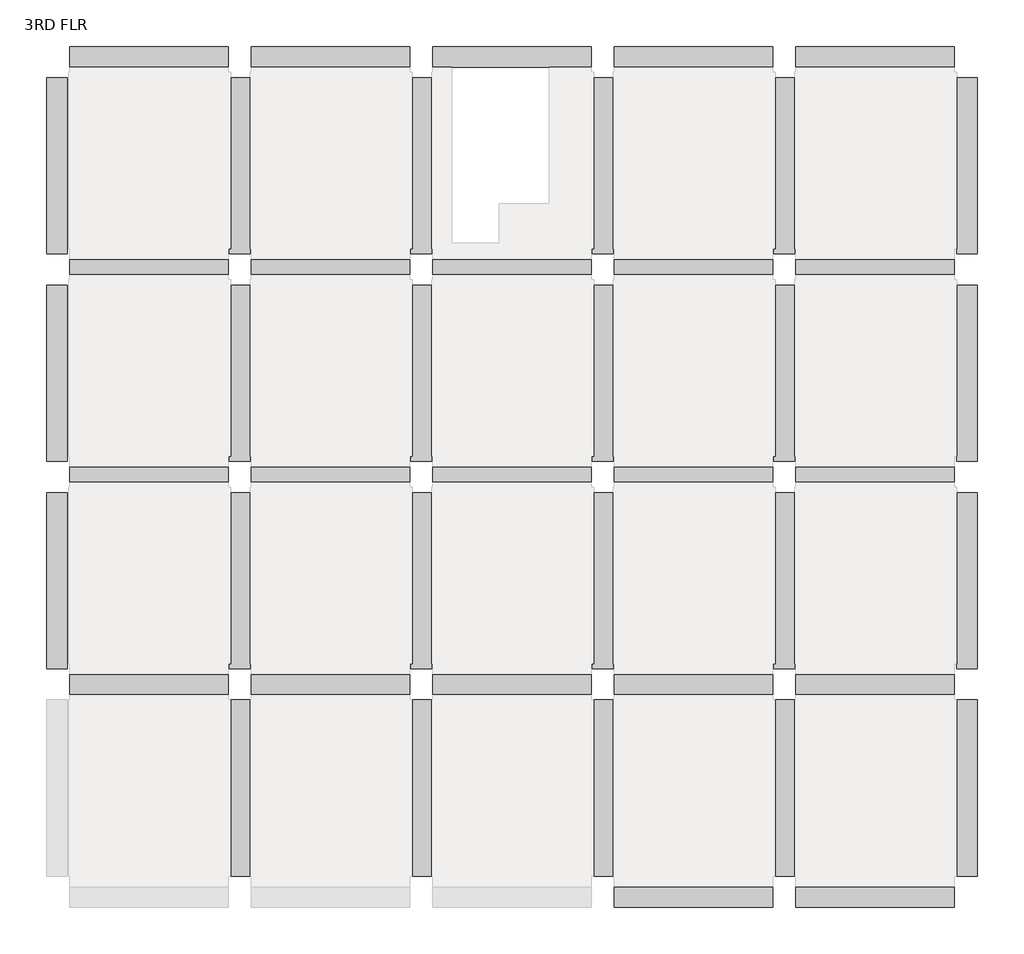
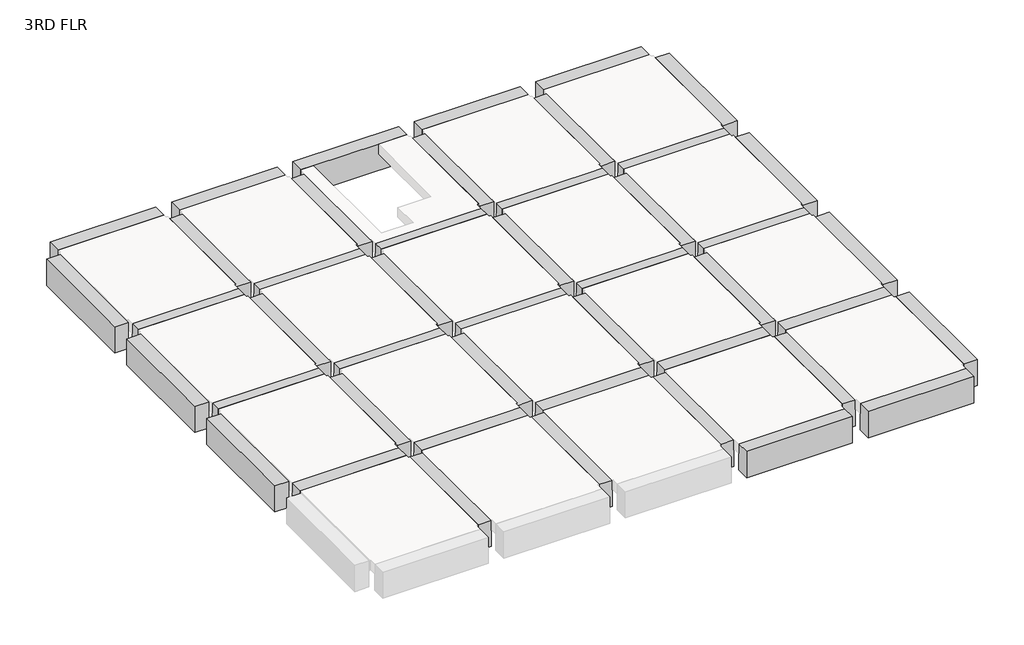
# One storey, part 2 of 2: 45 beams.
"""IFC4 building model written with IfcOpenShell, lengths in millimetres."""

from ifc_helpers import new_model, si_unit, frame, origin, place, context, project, spatial, polyline, outline, extrude, faceted_brep, element, save

model = new_model("IFC4")

# Units and contexts
model_context = context("Model", 3, world=origin())
ifc_project = project(units=[si_unit("LENGTHUNIT", "METRE", prefix="MILLI")], contexts=[model_context])

# Site, building, storey
site = spatial("IfcSite", under=ifc_project)
building = spatial("IfcBuilding", under=site)
storey = spatial("IfcBuildingStorey", under=building, Name="3RD FLR", Elevation=9144.0)

# Beams
placement = place(None, origin())
element("IfcBeam", 1, ObjectType="M_Concrete-Rectangular Beam : 400 x 800mm", at=placement, inside=storey, context=model_context, shape_type="Brep", body=[
    faceted_brep([(7955.1115906, 15703.1212443, 9144.0), (8355.1115906, 15703.1212443, 9144.0), (8355.1115906, 19103.1212443, 9144.0), (7955.1115906, 19103.1212443, 9144.0), (7955.1115906, 15803.1212443, 9144.0), (7955.1115906, 15703.1212443, 8344.0), (7955.1115906, 19103.1212443, 8344.0), (8355.1115906, 15703.1212443, 8344.0), (8355.1115906, 19103.1212443, 8344.0)], [[[0, 1, 2, 3, 4]], [[5, 0, 4, 3, 6]], [[7, 5, 6, 8]], [[1, 7, 8, 2]], [[2, 8, 6, 3]], [[1, 0, 5, 7]]]),
])
element("IfcBeam", 2, ObjectType="M_Concrete-Rectangular Beam : 400 x 800mm", at=placement, inside=storey, context=model_context, shape_type="Brep", body=[
    faceted_brep([(7955.1115906, 11703.1212443, 9144.0), (8355.1115906, 11703.1212443, 9144.0), (8355.1115906, 15103.1212443, 9144.0), (7955.1115906, 15103.1212443, 9144.0), (7955.1115906, 11803.1212443, 9144.0), (7955.1115906, 11703.1212443, 8344.0), (7955.1115906, 15103.1212443, 8344.0), (8355.1115906, 11703.1212443, 8344.0), (8355.1115906, 15103.1212443, 8344.0)], [[[0, 1, 2, 3, 4]], [[5, 0, 4, 3, 6]], [[7, 5, 6, 8]], [[1, 7, 8, 2]], [[2, 8, 6, 3]], [[1, 0, 5, 7]]]),
])
element("IfcBeam", 3, ObjectType="M_Concrete-Rectangular Beam : 400 x 800mm", at=placement, inside=storey, context=model_context, shape_type="Brep", body=[
    faceted_brep([(7955.1115906, 7703.1212443, 9144.0), (8355.1115906, 7703.1212443, 9144.0), (8355.1115906, 11103.1212443, 9144.0), (7955.1115906, 11103.1212443, 9144.0), (7955.1115906, 7803.1212443, 9144.0), (7955.1115906, 7703.1212443, 8344.0), (7955.1115906, 11103.1212443, 8344.0), (8355.1115906, 7703.1212443, 8344.0), (8355.1115906, 11103.1212443, 8344.0)], [[[0, 1, 2, 3, 4]], [[5, 0, 4, 3, 6]], [[7, 5, 6, 8]], [[1, 7, 8, 2]], [[1, 0, 5, 7]], [[3, 2, 8, 6]]]),
])
element("IfcBeam", 4, ObjectType="M_Concrete-Rectangular Beam : 400 x 800mm", at=placement, inside=storey, context=model_context, shape_type="Brep", body=[
    faceted_brep([(8355.1115906, 7103.1212443, 9144.0), (7955.1115906, 7103.1212443, 9144.0), (7955.1115906, 3703.1212443, 9144.0), (8355.1115906, 3703.1212443, 9144.0), (7955.1115906, 7103.1212443, 8844.0), (7955.1115906, 7103.1212443, 8344.0), (7955.1115906, 3703.1212443, 8344.0), (7955.1115906, 3703.1212443, 8844.0), (8355.1115906, 7103.1212443, 8344.0), (8355.1115906, 3703.1212443, 8344.0)], [[[0, 1, 2, 3]], [[1, 4, 5, 6, 7, 2]], [[5, 8, 9, 6]], [[8, 0, 3, 9]], [[0, 8, 5, 4, 1]], [[3, 2, 7, 6, 9]]]),
])
element("IfcBeam", 5, ObjectType="M_Concrete-Rectangular Beam : 400 x 800mm", at=placement, inside=storey, context=model_context, shape_type="Brep", body=[
    faceted_brep([(4855.1115906, 3503.1212443, 9144.0), (4855.1115906, 3103.1212443, 9144.0), (7905.1115906, 3103.1212443, 9144.0), (7905.1115906, 3503.1212443, 9144.0), (4855.1115906, 3503.1212443, 8344.0), (4855.1115906, 3503.1212443, 8844.0), (7905.1115906, 3503.1212443, 8844.0), (7905.1115906, 3503.1212443, 8344.0), (4855.1115906, 3103.1212443, 8344.0), (7905.1115906, 3103.1212443, 8344.0)], [[[0, 1, 2, 3]], [[4, 5, 0, 3, 6, 7]], [[8, 4, 7, 9]], [[1, 8, 9, 2]], [[1, 0, 5, 4, 8]], [[3, 2, 9, 7, 6]]]),
])
element("IfcBeam", 6, ObjectType="M_Concrete-Rectangular Beam : 400 x 800mm", at=placement, inside=storey, context=model_context, shape_type="Brep", body=[
    faceted_brep([(1355.1115906, 3503.1212443, 9144.0), (1355.1115906, 3103.1212443, 9144.0), (4405.1115906, 3103.1212443, 9144.0), (4405.1115906, 3503.1212443, 9144.0), (1355.1115906, 3503.1212443, 8344.0), (1355.1115906, 3503.1212443, 8844.0), (4405.1115906, 3503.1212443, 8844.0), (4405.1115906, 3503.1212443, 8344.0), (1355.1115906, 3103.1212443, 8344.0), (4405.1115906, 3103.1212443, 8344.0)], [[[0, 1, 2, 3]], [[4, 5, 0, 3, 6, 7]], [[8, 4, 7, 9]], [[1, 8, 9, 2]], [[1, 0, 5, 4, 8]], [[3, 2, 9, 7, 6]]]),
])
element("IfcBeam", 7, ObjectType="M_Concrete-Rectangular Beam : 400 x 800mm", at=placement, inside=storey, context=model_context, shape_type="SweptSolid", body=[
    extrude(outline(polyline([(-9594.8884094, 11103.1212443), (-9194.8884094, 11103.1212443), (-9194.8884094, 7703.1212443), (-9594.8884094, 7703.1212443), (-9594.8884094, 11103.1212443)])), frame((0.0, 0.0, 8344.0), z_axis=(0.0, 0.0, 1.0), x_axis=(1.0, 0.0, 0.0)), (0.0, 0.0, 1.0), 800.0),
])
element("IfcBeam", 8, ObjectType="M_Concrete-Rectangular Beam : 400 x 800mm", at=placement, inside=storey, context=model_context, shape_type="SweptSolid", body=[
    extrude(outline(polyline([(-9594.8884094, 15103.1212443), (-9194.8884094, 15103.1212443), (-9194.8884094, 11703.1212443), (-9594.8884094, 11703.1212443), (-9594.8884094, 15103.1212443)])), frame((0.0, 0.0, 8344.0), z_axis=(0.0, 0.0, 1.0), x_axis=(1.0, 0.0, 0.0)), (0.0, 0.0, 1.0), 800.0),
])
element("IfcBeam", 9, ObjectType="M_Concrete-Rectangular Beam : 400 x 800mm", at=placement, inside=storey, context=model_context, shape_type="Brep", body=[
    faceted_brep([(-2594.8884094, 19303.1212443, 9144.0), (-2594.8884094, 19703.1212443, 9144.0), (-5644.8884094, 19703.1212443, 9144.0), (-5644.8884094, 19303.1212443, 9144.0), (-2594.8884094, 19303.1212443, 8344.0), (-2594.8884094, 19303.1212443, 8844.0), (-5644.8884094, 19303.1212443, 8844.0), (-5644.8884094, 19303.1212443, 8344.0), (-2594.8884094, 19703.1212443, 8344.0), (-5644.8884094, 19703.1212443, 8344.0)], [[[0, 1, 2, 3]], [[4, 5, 0, 3, 6, 7]], [[8, 4, 7, 9]], [[1, 8, 9, 2]], [[1, 0, 5, 4, 8]], [[3, 2, 9, 7, 6]]]),
])
element("IfcBeam", 10, ObjectType="M_Concrete-Rectangular Beam : 400 x 800mm", at=placement, inside=storey, context=model_context, shape_type="Brep", body=[
    faceted_brep([(-2144.8884094, 19703.1212443, 9144.0), (-2144.8884094, 19303.1212443, 9144.0), (-1784.8884094, 19303.1212443, 9144.0), (94.7115906, 19303.1212443, 9144.0), (905.1115906, 19303.1212443, 9144.0), (905.1115906, 19703.1212443, 9144.0), (-2144.8884094, 19303.1212443, 8844.0), (-2144.8884094, 19303.1212443, 8344.0), (905.1115906, 19303.1212443, 8344.0), (905.1115906, 19303.1212443, 8844.0), (-2144.8884094, 19703.1212443, 8344.0), (905.1115906, 19703.1212443, 8344.0)], [[[0, 1, 2, 3, 4, 5]], [[1, 6, 7, 8, 9, 4, 3, 2]], [[7, 10, 11, 8]], [[10, 0, 5, 11]], [[1, 0, 10, 7, 6]], [[5, 4, 9, 8, 11]]]),
])
element("IfcBeam", 11, ObjectType="M_Concrete-Rectangular Beam : 400 x 800mm", at=placement, inside=storey, context=model_context, shape_type="Brep", body=[
    faceted_brep([(1355.1115906, 19703.1212443, 9144.0), (1355.1115906, 19303.1212443, 9144.0), (4405.1115906, 19303.1212443, 9144.0), (4405.1115906, 19703.1212443, 9144.0), (1355.1115906, 19303.1212443, 8844.0), (1355.1115906, 19303.1212443, 8344.0), (4405.1115906, 19303.1212443, 8344.0), (4405.1115906, 19303.1212443, 8844.0), (1355.1115906, 19703.1212443, 8344.0), (4405.1115906, 19703.1212443, 8344.0)], [[[0, 1, 2, 3]], [[1, 4, 5, 6, 7, 2]], [[5, 8, 9, 6]], [[8, 0, 3, 9]], [[1, 0, 8, 5, 4]], [[3, 2, 7, 6, 9]]]),
])
element("IfcBeam", 12, ObjectType="M_Concrete-Rectangular Beam : 400 x 800mm", at=placement, inside=storey, context=model_context, shape_type="Brep", body=[
    faceted_brep([(4855.1115906, 19703.1212443, 9144.0), (4855.1115906, 19303.1212443, 9144.0), (7905.1115906, 19303.1212443, 9144.0), (7905.1115906, 19703.1212443, 9144.0), (4855.1115906, 19303.1212443, 8844.0), (4855.1115906, 19303.1212443, 8344.0), (7905.1115906, 19303.1212443, 8344.0), (7905.1115906, 19303.1212443, 8844.0), (4855.1115906, 19703.1212443, 8344.0), (7905.1115906, 19703.1212443, 8344.0)], [[[0, 1, 2, 3]], [[1, 4, 5, 6, 7, 2]], [[5, 8, 9, 6]], [[8, 0, 3, 9]], [[1, 0, 8, 5, 4]], [[3, 2, 7, 6, 9]]]),
])
element("IfcBeam", 13, ObjectType="M_Concrete-Rectangular Beam : 400 x 800mm", at=placement, inside=storey, context=model_context, shape_type="Brep", body=[
    faceted_brep([(-5669.8884094, 15703.1212443, 9144.0), (-5669.8884094, 15803.1212443, 9144.0), (-5669.8884094, 19103.1212443, 9144.0), (-6044.8884094, 19103.1212443, 9144.0), (-6044.8884094, 15803.1212443, 9144.0), (-6069.8884094, 15803.1212443, 9144.0), (-6069.8884094, 15703.1212443, 9144.0), (-6069.8884094, 19103.1212443, 8344.0), (-6069.8884094, 15703.1212443, 8344.0), (-6069.8884094, 15803.1212443, 8844.0), (-6069.8884094, 19103.1212443, 8844.0), (-5669.8884094, 19103.1212443, 8344.0), (-5669.8884094, 15703.1212443, 8344.0), (-6044.8884094, 19103.1212443, 8844.0), (-6044.8884094, 15803.1212443, 8844.0)], [[[0, 1, 2, 3, 4, 5, 6]], [[7, 8, 6, 5, 9, 10]], [[7, 11, 12, 8]], [[11, 2, 1, 0, 12]], [[11, 7, 10, 13, 3, 2]], [[0, 6, 8, 12]], [[9, 14, 13, 10]], [[14, 4, 3, 13]], [[4, 14, 9, 5]]]),
])
element("IfcBeam", 14, ObjectType="M_Concrete-Rectangular Beam : 400 x 800mm", at=placement, inside=storey, context=model_context, shape_type="Brep", body=[
    faceted_brep([(-5669.8884094, 11703.1212443, 9144.0), (-5669.8884094, 11803.1212443, 9144.0), (-5669.8884094, 15103.1212443, 9144.0), (-6044.8884094, 15103.1212443, 9144.0), (-6044.8884094, 11803.1212443, 9144.0), (-6069.8884094, 11803.1212443, 9144.0), (-6069.8884094, 11703.1212443, 9144.0), (-6069.8884094, 15103.1212443, 8344.0), (-6069.8884094, 11703.1212443, 8344.0), (-6069.8884094, 11803.1212443, 8844.0), (-6069.8884094, 15103.1212443, 8844.0), (-5669.8884094, 15103.1212443, 8344.0), (-5669.8884094, 11703.1212443, 8344.0), (-6044.8884094, 15103.1212443, 8844.0), (-6044.8884094, 11803.1212443, 8844.0)], [[[0, 1, 2, 3, 4, 5, 6]], [[7, 8, 6, 5, 9, 10]], [[7, 11, 12, 8]], [[11, 2, 1, 0, 12]], [[11, 7, 10, 13, 3, 2]], [[0, 6, 8, 12]], [[9, 14, 13, 10]], [[14, 4, 3, 13]], [[4, 14, 9, 5]]]),
])
element("IfcBeam", 15, ObjectType="M_Concrete-Rectangular Beam : 400 x 800mm", at=placement, inside=storey, context=model_context, shape_type="Brep", body=[
    faceted_brep([(-5669.8884094, 7703.1212443, 9144.0), (-5669.8884094, 7803.1212443, 9144.0), (-5669.8884094, 11103.1212443, 9144.0), (-6044.8884094, 11103.1212443, 9144.0), (-6044.8884094, 7803.1212443, 9144.0), (-6069.8884094, 7803.1212443, 9144.0), (-6069.8884094, 7703.1212443, 9144.0), (-6069.8884094, 11103.1212443, 8344.0), (-6069.8884094, 7703.1212443, 8344.0), (-6069.8884094, 7803.1212443, 8844.0), (-6069.8884094, 11103.1212443, 8844.0), (-5669.8884094, 11103.1212443, 8344.0), (-5669.8884094, 7703.1212443, 8344.0), (-6044.8884094, 11103.1212443, 8844.0), (-6044.8884094, 7803.1212443, 8844.0)], [[[0, 1, 2, 3, 4, 5, 6]], [[7, 8, 6, 5, 9, 10]], [[8, 7, 11, 12]], [[2, 1, 0, 12, 11]], [[2, 11, 7, 10, 13, 3]], [[0, 6, 8, 12]], [[9, 14, 13, 10]], [[14, 4, 3, 13]], [[4, 14, 9, 5]]]),
])
element("IfcBeam", 16, ObjectType="M_Concrete-Rectangular Beam : 400 x 800mm", at=placement, inside=storey, context=model_context, shape_type="Brep", body=[
    faceted_brep([(-5669.8884094, 3703.1212443, 9144.0), (-5669.8884094, 7103.1212443, 9144.0), (-6044.8884094, 7103.1212443, 9144.0), (-6044.8884094, 3703.1212443, 9144.0), (-6069.8884094, 7103.1212443, 8344.0), (-6069.8884094, 3703.1212443, 8344.0), (-6069.8884094, 3703.1212443, 8844.0), (-6069.8884094, 7103.1212443, 8844.0), (-5669.8884094, 7103.1212443, 8344.0), (-5669.8884094, 3703.1212443, 8344.0), (-5669.8884094, 7103.1212443, 8844.0), (-5669.8884094, 3703.1212443, 8844.0), (-6044.8884094, 7103.1212443, 8844.0), (-6044.8884094, 3703.1212443, 8844.0)], [[[0, 1, 2, 3]], [[4, 5, 6, 7]], [[4, 8, 9, 5]], [[8, 10, 1, 0, 11, 9]], [[8, 4, 7, 12, 2, 1, 10]], [[5, 9, 11, 0, 3, 13, 6]], [[13, 12, 7, 6]], [[12, 13, 3, 2]]]),
])
element("IfcBeam", 17, ObjectType="M_Concrete-Rectangular Beam : 400 x 800mm", at=placement, inside=storey, context=model_context, shape_type="Brep", body=[
    faceted_brep([(-2169.8884094, 15703.1212443, 9144.0), (-2169.8884094, 15803.1212443, 9144.0), (-2169.8884094, 19103.1212443, 9144.0), (-2544.8884094, 19103.1212443, 9144.0), (-2544.8884094, 15803.1212443, 9144.0), (-2569.8884094, 15803.1212443, 9144.0), (-2569.8884094, 15703.1212443, 9144.0), (-2569.8884094, 19103.1212443, 8344.0), (-2569.8884094, 15703.1212443, 8344.0), (-2569.8884094, 15803.1212443, 8844.0), (-2569.8884094, 19103.1212443, 8844.0), (-2169.8884094, 19103.1212443, 8344.0), (-2169.8884094, 15703.1212443, 8344.0), (-2544.8884094, 19103.1212443, 8844.0), (-2544.8884094, 15803.1212443, 8844.0)], [[[0, 1, 2, 3, 4, 5, 6]], [[7, 8, 6, 5, 9, 10]], [[7, 11, 12, 8]], [[11, 2, 1, 0, 12]], [[11, 7, 10, 13, 3, 2]], [[0, 6, 8, 12]], [[9, 14, 13, 10]], [[14, 4, 3, 13]], [[4, 14, 9, 5]]]),
])
element("IfcBeam", 18, ObjectType="M_Concrete-Rectangular Beam : 400 x 800mm", at=placement, inside=storey, context=model_context, shape_type="Brep", body=[
    faceted_brep([(-2169.8884094, 11703.1212443, 9144.0), (-2169.8884094, 11803.1212443, 9144.0), (-2169.8884094, 15103.1212443, 9144.0), (-2544.8884094, 15103.1212443, 9144.0), (-2544.8884094, 11803.1212443, 9144.0), (-2569.8884094, 11803.1212443, 9144.0), (-2569.8884094, 11703.1212443, 9144.0), (-2569.8884094, 15103.1212443, 8344.0), (-2569.8884094, 11703.1212443, 8344.0), (-2569.8884094, 11803.1212443, 8844.0), (-2569.8884094, 15103.1212443, 8844.0), (-2169.8884094, 15103.1212443, 8344.0), (-2169.8884094, 11703.1212443, 8344.0), (-2544.8884094, 15103.1212443, 8844.0), (-2544.8884094, 11803.1212443, 8844.0)], [[[0, 1, 2, 3, 4, 5, 6]], [[7, 8, 6, 5, 9, 10]], [[8, 7, 11, 12]], [[2, 1, 0, 12, 11]], [[2, 11, 7, 10, 13, 3]], [[0, 6, 8, 12]], [[9, 14, 13, 10]], [[14, 4, 3, 13]], [[4, 14, 9, 5]]]),
])
element("IfcBeam", 19, ObjectType="M_Concrete-Rectangular Beam : 400 x 800mm", at=placement, inside=storey, context=model_context, shape_type="Brep", body=[
    faceted_brep([(-2169.8884094, 7703.1212443, 9144.0), (-2169.8884094, 7803.1212443, 9144.0), (-2169.8884094, 11103.1212443, 9144.0), (-2544.8884094, 11103.1212443, 9144.0), (-2544.8884094, 7803.1212443, 9144.0), (-2569.8884094, 7803.1212443, 9144.0), (-2569.8884094, 7703.1212443, 9144.0), (-2569.8884094, 11103.1212443, 8344.0), (-2569.8884094, 7703.1212443, 8344.0), (-2569.8884094, 7803.1212443, 8844.0), (-2569.8884094, 11103.1212443, 8844.0), (-2169.8884094, 11103.1212443, 8344.0), (-2169.8884094, 7703.1212443, 8344.0), (-2544.8884094, 11103.1212443, 8844.0), (-2544.8884094, 7803.1212443, 8844.0)], [[[0, 1, 2, 3, 4, 5, 6]], [[7, 8, 6, 5, 9, 10]], [[7, 11, 12, 8]], [[11, 2, 1, 0, 12]], [[2, 11, 7, 10, 13, 3]], [[0, 6, 8, 12]], [[9, 14, 13, 10]], [[14, 4, 3, 13]], [[4, 14, 9, 5]]]),
])
element("IfcBeam", 20, ObjectType="M_Concrete-Rectangular Beam : 400 x 800mm", at=placement, inside=storey, context=model_context, shape_type="Brep", body=[
    faceted_brep([(-2169.8884094, 3703.1212443, 9144.0), (-2169.8884094, 7103.1212443, 9144.0), (-2544.8884094, 7103.1212443, 9144.0), (-2544.8884094, 3703.1212443, 9144.0), (-2569.8884094, 7103.1212443, 8344.0), (-2569.8884094, 3703.1212443, 8344.0), (-2569.8884094, 3703.1212443, 8844.0), (-2569.8884094, 7103.1212443, 8844.0), (-2169.8884094, 7103.1212443, 8344.0), (-2169.8884094, 3703.1212443, 8344.0), (-2169.8884094, 7103.1212443, 8844.0), (-2169.8884094, 3703.1212443, 8844.0), (-2544.8884094, 7103.1212443, 8844.0), (-2544.8884094, 3703.1212443, 8844.0)], [[[0, 1, 2, 3]], [[4, 5, 6, 7]], [[4, 8, 9, 5]], [[8, 10, 1, 0, 11, 9]], [[8, 4, 7, 12, 2, 1, 10]], [[5, 9, 11, 0, 3, 13, 6]], [[13, 12, 7, 6]], [[12, 13, 3, 2]]]),
])
element("IfcBeam", 21, ObjectType="M_Concrete-Rectangular Beam : 400 x 800mm", at=placement, inside=storey, context=model_context, shape_type="Brep", body=[
    faceted_brep([(1330.1115906, 15703.1212443, 9144.0), (1330.1115906, 15803.1212443, 9144.0), (1330.1115906, 19103.1212443, 9144.0), (955.1115906, 19103.1212443, 9144.0), (955.1115906, 15803.1212443, 9144.0), (930.1115906, 15803.1212443, 9144.0), (930.1115906, 15703.1212443, 9144.0), (930.1115906, 19103.1212443, 8344.0), (930.1115906, 15703.1212443, 8344.0), (930.1115906, 15803.1212443, 8844.0), (930.1115906, 19103.1212443, 8844.0), (1330.1115906, 19103.1212443, 8344.0), (1330.1115906, 15703.1212443, 8344.0), (955.1115906, 19103.1212443, 8844.0), (955.1115906, 15803.1212443, 8844.0)], [[[0, 1, 2, 3, 4, 5, 6]], [[7, 8, 6, 5, 9, 10]], [[7, 11, 12, 8]], [[11, 2, 1, 0, 12]], [[2, 11, 7, 10, 13, 3]], [[0, 6, 8, 12]], [[9, 14, 13, 10]], [[14, 4, 3, 13]], [[4, 14, 9, 5]]]),
])
element("IfcBeam", 22, ObjectType="M_Concrete-Rectangular Beam : 400 x 800mm", at=placement, inside=storey, context=model_context, shape_type="Brep", body=[
    faceted_brep([(1330.1115906, 11703.1212443, 9144.0), (1330.1115906, 11803.1212443, 9144.0), (1330.1115906, 15103.1212443, 9144.0), (955.1115906, 15103.1212443, 9144.0), (955.1115906, 11803.1212443, 9144.0), (930.1115906, 11803.1212443, 9144.0), (930.1115906, 11703.1212443, 9144.0), (930.1115906, 15103.1212443, 8344.0), (930.1115906, 11703.1212443, 8344.0), (930.1115906, 11803.1212443, 8844.0), (930.1115906, 15103.1212443, 8844.0), (1330.1115906, 15103.1212443, 8344.0), (1330.1115906, 11703.1212443, 8344.0), (955.1115906, 15103.1212443, 8844.0), (955.1115906, 11803.1212443, 8844.0)], [[[0, 1, 2, 3, 4, 5, 6]], [[7, 8, 6, 5, 9, 10]], [[8, 7, 11, 12]], [[2, 1, 0, 12, 11]], [[2, 11, 7, 10, 13, 3]], [[0, 6, 8, 12]], [[9, 14, 13, 10]], [[14, 4, 3, 13]], [[4, 14, 9, 5]]]),
])
element("IfcBeam", 23, ObjectType="M_Concrete-Rectangular Beam : 400 x 800mm", at=placement, inside=storey, context=model_context, shape_type="Brep", body=[
    faceted_brep([(1330.1115906, 7703.1212443, 9144.0), (1330.1115906, 7803.1212443, 9144.0), (1330.1115906, 11103.1212443, 9144.0), (955.1115906, 11103.1212443, 9144.0), (955.1115906, 7803.1212443, 9144.0), (930.1115906, 7803.1212443, 9144.0), (930.1115906, 7703.1212443, 9144.0), (930.1115906, 11103.1212443, 8344.0), (930.1115906, 7703.1212443, 8344.0), (930.1115906, 7803.1212443, 8844.0), (930.1115906, 11103.1212443, 8844.0), (1330.1115906, 11103.1212443, 8344.0), (1330.1115906, 7703.1212443, 8344.0), (955.1115906, 11103.1212443, 8844.0), (955.1115906, 7803.1212443, 8844.0)], [[[0, 1, 2, 3, 4, 5, 6]], [[7, 8, 6, 5, 9, 10]], [[7, 11, 12, 8]], [[11, 2, 1, 0, 12]], [[2, 11, 7, 10, 13, 3]], [[0, 6, 8, 12]], [[9, 14, 13, 10]], [[14, 4, 3, 13]], [[4, 14, 9, 5]]]),
])
element("IfcBeam", 24, ObjectType="M_Concrete-Rectangular Beam : 400 x 800mm", at=placement, inside=storey, context=model_context, shape_type="Brep", body=[
    faceted_brep([(1330.1115906, 3703.1212443, 9144.0), (1330.1115906, 7103.1212443, 9144.0), (955.1115906, 7103.1212443, 9144.0), (955.1115906, 3703.1212443, 9144.0), (930.1115906, 7103.1212443, 8344.0), (930.1115906, 3703.1212443, 8344.0), (930.1115906, 3703.1212443, 8844.0), (930.1115906, 7103.1212443, 8844.0), (1330.1115906, 7103.1212443, 8344.0), (1330.1115906, 3703.1212443, 8344.0), (1330.1115906, 7103.1212443, 8844.0), (1330.1115906, 3703.1212443, 8844.0), (955.1115906, 7103.1212443, 8844.0), (955.1115906, 3703.1212443, 8844.0)], [[[0, 1, 2, 3]], [[4, 5, 6, 7]], [[4, 8, 9, 5]], [[8, 10, 1, 0, 11, 9]], [[8, 4, 7, 12, 2, 1, 10]], [[5, 9, 11, 0, 3, 13, 6]], [[13, 12, 7, 6]], [[12, 13, 3, 2]]]),
])
element("IfcBeam", 25, ObjectType="M_Concrete-Rectangular Beam : 400 x 800mm", at=placement, inside=storey, context=model_context, shape_type="Brep", body=[
    faceted_brep([(4830.1115906, 15703.1212443, 9144.0), (4830.1115906, 15803.1212443, 9144.0), (4830.1115906, 19103.1212443, 9144.0), (4455.1115906, 19103.1212443, 9144.0), (4455.1115906, 15803.1212443, 9144.0), (4430.1115906, 15803.1212443, 9144.0), (4430.1115906, 15703.1212443, 9144.0), (4430.1115906, 19103.1212443, 8344.0), (4430.1115906, 15703.1212443, 8344.0), (4430.1115906, 15803.1212443, 8844.0), (4430.1115906, 19103.1212443, 8844.0), (4830.1115906, 19103.1212443, 8344.0), (4830.1115906, 15703.1212443, 8344.0), (4455.1115906, 19103.1212443, 8844.0), (4455.1115906, 15803.1212443, 8844.0)], [[[0, 1, 2, 3, 4, 5, 6]], [[7, 8, 6, 5, 9, 10]], [[8, 7, 11, 12]], [[2, 1, 0, 12, 11]], [[2, 11, 7, 10, 13, 3]], [[0, 6, 8, 12]], [[9, 14, 13, 10]], [[14, 4, 3, 13]], [[4, 14, 9, 5]]]),
])
element("IfcBeam", 26, ObjectType="M_Concrete-Rectangular Beam : 400 x 800mm", at=placement, inside=storey, context=model_context, shape_type="Brep", body=[
    faceted_brep([(4830.1115906, 11703.1212443, 9144.0), (4830.1115906, 11803.1212443, 9144.0), (4830.1115906, 15103.1212443, 9144.0), (4455.1115906, 15103.1212443, 9144.0), (4455.1115906, 11803.1212443, 9144.0), (4430.1115906, 11803.1212443, 9144.0), (4430.1115906, 11703.1212443, 9144.0), (4430.1115906, 15103.1212443, 8344.0), (4430.1115906, 11703.1212443, 8344.0), (4430.1115906, 11803.1212443, 8844.0), (4430.1115906, 15103.1212443, 8844.0), (4830.1115906, 15103.1212443, 8344.0), (4830.1115906, 11703.1212443, 8344.0), (4455.1115906, 15103.1212443, 8844.0), (4455.1115906, 11803.1212443, 8844.0)], [[[0, 1, 2, 3, 4, 5, 6]], [[7, 8, 6, 5, 9, 10]], [[7, 11, 12, 8]], [[11, 2, 1, 0, 12]], [[2, 11, 7, 10, 13, 3]], [[0, 6, 8, 12]], [[9, 14, 13, 10]], [[14, 4, 3, 13]], [[4, 14, 9, 5]]]),
])
element("IfcBeam", 27, ObjectType="M_Concrete-Rectangular Beam : 400 x 800mm", at=placement, inside=storey, context=model_context, shape_type="Brep", body=[
    faceted_brep([(4430.1115906, 7703.1212443, 9144.0), (4830.1115906, 7703.1212443, 9144.0), (4830.1115906, 7803.1212443, 9144.0), (4830.1115906, 11103.1212443, 9144.0), (4455.1115906, 11103.1212443, 9144.0), (4455.1115906, 7803.1212443, 9144.0), (4430.1115906, 7803.1212443, 9144.0), (4430.1115906, 7703.1212443, 8344.0), (4430.1115906, 7803.1212443, 8844.0), (4430.1115906, 11103.1212443, 8844.0), (4430.1115906, 11103.1212443, 8344.0), (4830.1115906, 7703.1212443, 8344.0), (4830.1115906, 11103.1212443, 8344.0), (4455.1115906, 11103.1212443, 8844.0), (4455.1115906, 7803.1212443, 8844.0)], [[[0, 1, 2, 3, 4, 5, 6]], [[7, 0, 6, 8, 9, 10]], [[11, 7, 10, 12]], [[1, 11, 12, 3, 2]], [[1, 0, 7, 11]], [[12, 10, 9, 13, 4, 3]], [[8, 14, 13, 9]], [[14, 5, 4, 13]], [[5, 14, 8, 6]]]),
])
element("IfcBeam", 28, ObjectType="M_Concrete-Rectangular Beam : 400 x 800mm", at=placement, inside=storey, context=model_context, shape_type="Brep", body=[
    faceted_brep([(4830.1115906, 3703.1212443, 9144.0), (4830.1115906, 7103.1212443, 9144.0), (4455.1115906, 7103.1212443, 9144.0), (4455.1115906, 3703.1212443, 9144.0), (4430.1115906, 7103.1212443, 8344.0), (4430.1115906, 3703.1212443, 8344.0), (4430.1115906, 3703.1212443, 8844.0), (4430.1115906, 7103.1212443, 8844.0), (4830.1115906, 7103.1212443, 8344.0), (4830.1115906, 3703.1212443, 8344.0), (4830.1115906, 7103.1212443, 8844.0), (4830.1115906, 3703.1212443, 8844.0), (4455.1115906, 7103.1212443, 8844.0), (4455.1115906, 3703.1212443, 8844.0)], [[[0, 1, 2, 3]], [[4, 5, 6, 7]], [[4, 8, 9, 5]], [[8, 10, 1, 0, 11, 9]], [[1, 10, 8, 4, 7, 12, 2]], [[5, 9, 11, 0, 3, 13, 6]], [[13, 12, 7, 6]], [[12, 13, 3, 2]]]),
])
element("IfcBeam", 29, ObjectType="M_Concrete-Rectangular Beam : 400 x 800mm", at=placement, inside=storey, context=model_context, shape_type="Brep", body=[
    faceted_brep([(-6094.8884094, 15603.1212443, 9144.0), (-9144.8884094, 15603.1212443, 9144.0), (-9144.8884094, 15303.1212443, 9144.0), (-6094.8884094, 15303.1212443, 9144.0), (-9144.8884094, 15203.1212443, 8344.0), (-6094.8884094, 15203.1212443, 8344.0), (-6094.8884094, 15203.1212443, 8844.0), (-9144.8884094, 15203.1212443, 8844.0), (-9144.8884094, 15603.1212443, 8344.0), (-6094.8884094, 15603.1212443, 8344.0), (-9144.8884094, 15603.1212443, 8844.0), (-6094.8884094, 15603.1212443, 8844.0), (-9144.8884094, 15303.1212443, 8844.0), (-6094.8884094, 15303.1212443, 8844.0)], [[[0, 1, 2, 3]], [[4, 5, 6, 7]], [[4, 8, 9, 5]], [[8, 10, 1, 0, 11, 9]], [[8, 4, 7, 12, 2, 1, 10]], [[5, 9, 11, 0, 3, 13, 6]], [[13, 12, 7, 6]], [[12, 13, 3, 2]]]),
])
element("IfcBeam", 30, ObjectType="M_Concrete-Rectangular Beam : 400 x 800mm", at=placement, inside=storey, context=model_context, shape_type="Brep", body=[
    faceted_brep([(-2594.8884094, 15603.1212443, 9144.0), (-5644.8884094, 15603.1212443, 9144.0), (-5644.8884094, 15303.1212443, 9144.0), (-2594.8884094, 15303.1212443, 9144.0), (-5644.8884094, 15203.1212443, 8344.0), (-2594.8884094, 15203.1212443, 8344.0), (-2594.8884094, 15203.1212443, 8844.0), (-5644.8884094, 15203.1212443, 8844.0), (-5644.8884094, 15603.1212443, 8344.0), (-2594.8884094, 15603.1212443, 8344.0), (-5644.8884094, 15603.1212443, 8844.0), (-2594.8884094, 15603.1212443, 8844.0), (-5644.8884094, 15303.1212443, 8844.0), (-2594.8884094, 15303.1212443, 8844.0)], [[[0, 1, 2, 3]], [[4, 5, 6, 7]], [[4, 8, 9, 5]], [[8, 10, 1, 0, 11, 9]], [[8, 4, 7, 12, 2, 1, 10]], [[5, 9, 11, 0, 3, 13, 6]], [[13, 12, 7, 6]], [[12, 13, 3, 2]]]),
])
element("IfcBeam", 31, ObjectType="M_Concrete-Rectangular Beam : 400 x 800mm", at=placement, inside=storey, context=model_context, shape_type="Brep", body=[
    faceted_brep([(905.1115906, 15603.1212443, 9144.0), (-2144.8884094, 15603.1212443, 9144.0), (-2144.8884094, 15303.1212443, 9144.0), (905.1115906, 15303.1212443, 9144.0), (-2144.8884094, 15603.1212443, 8344.0), (-2144.8884094, 15603.1212443, 8844.0), (905.1115906, 15603.1212443, 8844.0), (905.1115906, 15603.1212443, 8344.0), (-2144.8884094, 15203.1212443, 8344.0), (905.1115906, 15203.1212443, 8344.0), (905.1115906, 15203.1212443, 8844.0), (-2144.8884094, 15203.1212443, 8844.0), (-2144.8884094, 15303.1212443, 8844.0), (905.1115906, 15303.1212443, 8844.0)], [[[0, 1, 2, 3]], [[4, 5, 1, 0, 6, 7]], [[8, 4, 7, 9]], [[8, 9, 10, 11]], [[1, 5, 4, 8, 11, 12, 2]], [[7, 6, 0, 3, 13, 10, 9]], [[13, 12, 11, 10]], [[12, 13, 3, 2]]]),
])
element("IfcBeam", 32, ObjectType="M_Concrete-Rectangular Beam : 400 x 800mm", at=placement, inside=storey, context=model_context, shape_type="Brep", body=[
    faceted_brep([(4405.1115906, 15603.1212443, 9144.0), (1355.1115906, 15603.1212443, 9144.0), (1355.1115906, 15303.1212443, 9144.0), (4405.1115906, 15303.1212443, 9144.0), (1355.1115906, 15203.1212443, 8344.0), (4405.1115906, 15203.1212443, 8344.0), (4405.1115906, 15203.1212443, 8844.0), (1355.1115906, 15203.1212443, 8844.0), (1355.1115906, 15603.1212443, 8344.0), (4405.1115906, 15603.1212443, 8344.0), (1355.1115906, 15603.1212443, 8844.0), (4405.1115906, 15603.1212443, 8844.0), (1355.1115906, 15303.1212443, 8844.0), (4405.1115906, 15303.1212443, 8844.0)], [[[0, 1, 2, 3]], [[4, 5, 6, 7]], [[4, 8, 9, 5]], [[8, 10, 1, 0, 11, 9]], [[8, 4, 7, 12, 2, 1, 10]], [[5, 9, 11, 0, 3, 13, 6]], [[13, 12, 7, 6]], [[12, 13, 3, 2]]]),
])
element("IfcBeam", 33, ObjectType="M_Concrete-Rectangular Beam : 400 x 800mm", at=placement, inside=storey, context=model_context, shape_type="Brep", body=[
    faceted_brep([(7905.1115906, 15603.1212443, 9144.0), (4855.1115906, 15603.1212443, 9144.0), (4855.1115906, 15303.1212443, 9144.0), (7905.1115906, 15303.1212443, 9144.0), (4855.1115906, 15203.1212443, 8344.0), (7905.1115906, 15203.1212443, 8344.0), (7905.1115906, 15203.1212443, 8844.0), (4855.1115906, 15203.1212443, 8844.0), (4855.1115906, 15603.1212443, 8344.0), (7905.1115906, 15603.1212443, 8344.0), (4855.1115906, 15603.1212443, 8844.0), (7905.1115906, 15603.1212443, 8844.0), (4855.1115906, 15303.1212443, 8844.0), (7905.1115906, 15303.1212443, 8844.0)], [[[0, 1, 2, 3]], [[4, 5, 6, 7]], [[4, 8, 9, 5]], [[8, 10, 1, 0, 11, 9]], [[8, 4, 7, 12, 2, 1, 10]], [[5, 9, 11, 0, 3, 13, 6]], [[13, 12, 7, 6]], [[12, 13, 3, 2]]]),
])
element("IfcBeam", 34, ObjectType="M_Concrete-Rectangular Beam : 400 x 800mm", at=placement, inside=storey, context=model_context, shape_type="Brep", body=[
    faceted_brep([(7905.1115906, 11603.1212443, 9144.0), (4855.1115906, 11603.1212443, 9144.0), (4855.1115906, 11303.1212443, 9144.0), (7905.1115906, 11303.1212443, 9144.0), (4855.1115906, 11603.1212443, 8344.0), (4855.1115906, 11603.1212443, 8844.0), (7905.1115906, 11603.1212443, 8844.0), (7905.1115906, 11603.1212443, 8344.0), (4855.1115906, 11203.1212443, 8344.0), (7905.1115906, 11203.1212443, 8344.0), (7905.1115906, 11203.1212443, 8844.0), (4855.1115906, 11203.1212443, 8844.0), (4855.1115906, 11303.1212443, 8844.0), (7905.1115906, 11303.1212443, 8844.0)], [[[0, 1, 2, 3]], [[4, 5, 1, 0, 6, 7]], [[8, 4, 7, 9]], [[8, 9, 10, 11]], [[1, 5, 4, 8, 11, 12, 2]], [[7, 6, 0, 3, 13, 10, 9]], [[13, 12, 11, 10]], [[12, 13, 3, 2]]]),
])
element("IfcBeam", 35, ObjectType="M_Concrete-Rectangular Beam : 400 x 800mm", at=placement, inside=storey, context=model_context, shape_type="Brep", body=[
    faceted_brep([(4405.1115906, 11603.1212443, 9144.0), (1355.1115906, 11603.1212443, 9144.0), (1355.1115906, 11303.1212443, 9144.0), (4405.1115906, 11303.1212443, 9144.0), (1355.1115906, 11603.1212443, 8344.0), (1355.1115906, 11603.1212443, 8844.0), (4405.1115906, 11603.1212443, 8844.0), (4405.1115906, 11603.1212443, 8344.0), (1355.1115906, 11203.1212443, 8344.0), (4405.1115906, 11203.1212443, 8344.0), (4405.1115906, 11203.1212443, 8844.0), (1355.1115906, 11203.1212443, 8844.0), (1355.1115906, 11303.1212443, 8844.0), (4405.1115906, 11303.1212443, 8844.0)], [[[0, 1, 2, 3]], [[4, 5, 1, 0, 6, 7]], [[8, 4, 7, 9]], [[8, 9, 10, 11]], [[1, 5, 4, 8, 11, 12, 2]], [[7, 6, 0, 3, 13, 10, 9]], [[13, 12, 11, 10]], [[12, 13, 3, 2]]]),
])
element("IfcBeam", 36, ObjectType="M_Concrete-Rectangular Beam : 400 x 800mm", at=placement, inside=storey, context=model_context, shape_type="Brep", body=[
    faceted_brep([(905.1115906, 11603.1212443, 9144.0), (-2144.8884094, 11603.1212443, 9144.0), (-2144.8884094, 11303.1212443, 9144.0), (905.1115906, 11303.1212443, 9144.0), (-2144.8884094, 11603.1212443, 8344.0), (-2144.8884094, 11603.1212443, 8844.0), (905.1115906, 11603.1212443, 8844.0), (905.1115906, 11603.1212443, 8344.0), (-2144.8884094, 11203.1212443, 8344.0), (905.1115906, 11203.1212443, 8344.0), (905.1115906, 11203.1212443, 8844.0), (-2144.8884094, 11203.1212443, 8844.0), (-2144.8884094, 11303.1212443, 8844.0), (905.1115906, 11303.1212443, 8844.0)], [[[0, 1, 2, 3]], [[4, 5, 1, 0, 6, 7]], [[8, 4, 7, 9]], [[8, 9, 10, 11]], [[1, 5, 4, 8, 11, 12, 2]], [[7, 6, 0, 3, 13, 10, 9]], [[13, 12, 11, 10]], [[12, 13, 3, 2]]]),
])
element("IfcBeam", 37, ObjectType="M_Concrete-Rectangular Beam : 400 x 800mm", at=placement, inside=storey, context=model_context, shape_type="Brep", body=[
    faceted_brep([(-2594.8884094, 11603.1212443, 9144.0), (-5644.8884094, 11603.1212443, 9144.0), (-5644.8884094, 11303.1212443, 9144.0), (-2594.8884094, 11303.1212443, 9144.0), (-5644.8884094, 11603.1212443, 8344.0), (-5644.8884094, 11603.1212443, 8844.0), (-2594.8884094, 11603.1212443, 8844.0), (-2594.8884094, 11603.1212443, 8344.0), (-5644.8884094, 11203.1212443, 8344.0), (-2594.8884094, 11203.1212443, 8344.0), (-2594.8884094, 11203.1212443, 8844.0), (-5644.8884094, 11203.1212443, 8844.0), (-5644.8884094, 11303.1212443, 8844.0), (-2594.8884094, 11303.1212443, 8844.0)], [[[0, 1, 2, 3]], [[4, 5, 1, 0, 6, 7]], [[8, 4, 7, 9]], [[8, 9, 10, 11]], [[1, 5, 4, 8, 11, 12, 2]], [[7, 6, 0, 3, 13, 10, 9]], [[13, 12, 11, 10]], [[12, 13, 3, 2]]]),
])
element("IfcBeam", 38, ObjectType="M_Concrete-Rectangular Beam : 400 x 800mm", at=placement, inside=storey, context=model_context, shape_type="Brep", body=[
    faceted_brep([(-6094.8884094, 11603.1212443, 9144.0), (-9144.8884094, 11603.1212443, 9144.0), (-9144.8884094, 11303.1212443, 9144.0), (-6094.8884094, 11303.1212443, 9144.0), (-9144.8884094, 11603.1212443, 8344.0), (-9144.8884094, 11603.1212443, 8844.0), (-6094.8884094, 11603.1212443, 8844.0), (-6094.8884094, 11603.1212443, 8344.0), (-9144.8884094, 11203.1212443, 8344.0), (-6094.8884094, 11203.1212443, 8344.0), (-6094.8884094, 11203.1212443, 8844.0), (-9144.8884094, 11203.1212443, 8844.0), (-9144.8884094, 11303.1212443, 8844.0), (-6094.8884094, 11303.1212443, 8844.0)], [[[0, 1, 2, 3]], [[4, 5, 1, 0, 6, 7]], [[8, 4, 7, 9]], [[8, 9, 10, 11]], [[1, 5, 4, 8, 11, 12, 2]], [[7, 6, 0, 3, 13, 10, 9]], [[13, 12, 11, 10]], [[12, 13, 3, 2]]]),
])
element("IfcBeam", 39, ObjectType="M_Concrete-Rectangular Beam : 400 x 800mm", at=placement, inside=storey, context=model_context, shape_type="Brep", body=[
    faceted_brep([(-9144.8884094, 7603.1212443, 9144.0), (-9144.8884094, 7203.1212443, 9144.0), (-6094.8884094, 7203.1212443, 9144.0), (-6094.8884094, 7603.1212443, 9144.0), (-9144.8884094, 7203.1212443, 8844.0), (-9144.8884094, 7203.1212443, 8344.0), (-6094.8884094, 7203.1212443, 8344.0), (-6094.8884094, 7203.1212443, 8844.0), (-9144.8884094, 7603.1212443, 8344.0), (-6094.8884094, 7603.1212443, 8344.0), (-9144.8884094, 7603.1212443, 8844.0), (-6094.8884094, 7603.1212443, 8844.0)], [[[0, 1, 2, 3]], [[1, 4, 5, 6, 7, 2]], [[5, 8, 9, 6]], [[8, 10, 0, 3, 11, 9]], [[1, 0, 10, 8, 5, 4]], [[3, 2, 7, 6, 9, 11]]]),
])
element("IfcBeam", 40, ObjectType="M_Concrete-Rectangular Beam : 400 x 800mm", at=placement, inside=storey, context=model_context, shape_type="Brep", body=[
    faceted_brep([(-5644.8884094, 7603.1212443, 9144.0), (-5644.8884094, 7203.1212443, 9144.0), (-2594.8884094, 7203.1212443, 9144.0), (-2594.8884094, 7603.1212443, 9144.0), (-5644.8884094, 7203.1212443, 8844.0), (-5644.8884094, 7203.1212443, 8344.0), (-2594.8884094, 7203.1212443, 8344.0), (-2594.8884094, 7203.1212443, 8844.0), (-5644.8884094, 7603.1212443, 8344.0), (-2594.8884094, 7603.1212443, 8344.0), (-5644.8884094, 7603.1212443, 8844.0), (-2594.8884094, 7603.1212443, 8844.0)], [[[0, 1, 2, 3]], [[1, 4, 5, 6, 7, 2]], [[5, 8, 9, 6]], [[8, 10, 0, 3, 11, 9]], [[1, 0, 10, 8, 5, 4]], [[3, 2, 7, 6, 9, 11]]]),
])
element("IfcBeam", 41, ObjectType="M_Concrete-Rectangular Beam : 400 x 800mm", at=placement, inside=storey, context=model_context, shape_type="Brep", body=[
    faceted_brep([(-2144.8884094, 7603.1212443, 9144.0), (-2144.8884094, 7203.1212443, 9144.0), (905.1115906, 7203.1212443, 9144.0), (905.1115906, 7603.1212443, 9144.0), (-2144.8884094, 7203.1212443, 8844.0), (-2144.8884094, 7203.1212443, 8344.0), (905.1115906, 7203.1212443, 8344.0), (905.1115906, 7203.1212443, 8844.0), (-2144.8884094, 7603.1212443, 8344.0), (905.1115906, 7603.1212443, 8344.0), (-2144.8884094, 7603.1212443, 8844.0), (905.1115906, 7603.1212443, 8844.0)], [[[0, 1, 2, 3]], [[1, 4, 5, 6, 7, 2]], [[5, 8, 9, 6]], [[8, 10, 0, 3, 11, 9]], [[1, 0, 10, 8, 5, 4]], [[3, 2, 7, 6, 9, 11]]]),
])
element("IfcBeam", 42, ObjectType="M_Concrete-Rectangular Beam : 400 x 800mm", at=placement, inside=storey, context=model_context, shape_type="Brep", body=[
    faceted_brep([(1355.1115906, 7603.1212443, 9144.0), (1355.1115906, 7203.1212443, 9144.0), (4405.1115906, 7203.1212443, 9144.0), (4405.1115906, 7603.1212443, 9144.0), (1355.1115906, 7203.1212443, 8844.0), (1355.1115906, 7203.1212443, 8344.0), (4405.1115906, 7203.1212443, 8344.0), (4405.1115906, 7203.1212443, 8844.0), (1355.1115906, 7603.1212443, 8344.0), (4405.1115906, 7603.1212443, 8344.0), (1355.1115906, 7603.1212443, 8844.0), (4405.1115906, 7603.1212443, 8844.0)], [[[0, 1, 2, 3]], [[1, 4, 5, 6, 7, 2]], [[5, 8, 9, 6]], [[8, 10, 0, 3, 11, 9]], [[1, 0, 10, 8, 5, 4]], [[3, 2, 7, 6, 9, 11]]]),
])
element("IfcBeam", 43, ObjectType="M_Concrete-Rectangular Beam : 400 x 800mm", at=placement, inside=storey, context=model_context, shape_type="Brep", body=[
    faceted_brep([(4855.1115906, 7603.1212443, 9144.0), (4855.1115906, 7203.1212443, 9144.0), (7905.1115906, 7203.1212443, 9144.0), (7905.1115906, 7603.1212443, 9144.0), (4855.1115906, 7203.1212443, 8844.0), (4855.1115906, 7203.1212443, 8344.0), (7905.1115906, 7203.1212443, 8344.0), (7905.1115906, 7203.1212443, 8844.0), (4855.1115906, 7603.1212443, 8344.0), (7905.1115906, 7603.1212443, 8344.0), (4855.1115906, 7603.1212443, 8844.0), (7905.1115906, 7603.1212443, 8844.0)], [[[0, 1, 2, 3]], [[1, 4, 5, 6, 7, 2]], [[5, 8, 9, 6]], [[8, 10, 0, 3, 11, 9]], [[1, 0, 10, 8, 5, 4]], [[3, 2, 7, 6, 9, 11]]]),
])
element("IfcBeam", 44, ObjectType="M_Concrete-Rectangular Beam : 400 x 800mm", at=placement, inside=storey, context=model_context, shape_type="SweptSolid", body=[
    extrude(outline(polyline([(-9594.8884094, 19103.1212443), (-9194.8884094, 19103.1212443), (-9194.8884094, 15703.1212443), (-9594.8884094, 15703.1212443), (-9594.8884094, 19103.1212443)])), frame((0.0, 0.0, 8344.0), z_axis=(0.0, 0.0, 1.0), x_axis=(1.0, 0.0, 0.0)), (0.0, 0.0, 1.0), 800.0),
])
element("IfcBeam", 45, ObjectType="M_Concrete-Rectangular Beam : 400 x 800mm", at=placement, inside=storey, context=model_context, shape_type="Brep", body=[
    faceted_brep([(-6094.8884094, 19303.1212443, 9144.0), (-6094.8884094, 19703.1212443, 9144.0), (-9144.8884094, 19703.1212443, 9144.0), (-9144.8884094, 19303.1212443, 9144.0), (-6094.8884094, 19303.1212443, 8344.0), (-6094.8884094, 19303.1212443, 8844.0), (-9144.8884094, 19303.1212443, 8844.0), (-9144.8884094, 19303.1212443, 8344.0), (-6094.8884094, 19703.1212443, 8344.0), (-9144.8884094, 19703.1212443, 8344.0)], [[[0, 1, 2, 3]], [[4, 5, 0, 3, 6, 7]], [[8, 4, 7, 9]], [[1, 8, 9, 2]], [[2, 9, 7, 6, 3]], [[1, 0, 5, 4, 8]]]),
])

save(model, "model.ifc")

# Revit data of these elements
# Type "M_Concrete-Rectangular Beam : 400 x 800mm"
#   Length [instance default] = 5' - 0"
#   b = 1' - 3.74803"
#   h = 2' - 7.49606"
#   Structural Material [instance default] = Concrete, Cast-in-Place gray
#   Assembly Code = ""
# Elements 1, 2, 3, 4, 5, 6, 7, 8, 9, 10, 11, 12, 13, 14, 15, 16, 17, 18, 19, 20, 21, 22, 23, 24, 25, 26, 27, 28, 29, 30, 31, 32, 33, 34, 35, 36, 37, 38, 39, 40, 41, 42, 43, 44, 45 (IfcBeam, "M_Concrete-Rectangular Beam : 400 x 800mm")
#   Structural Material = Concrete, Cast-in-Place gray
#   Phase Created = New Construction
#   Materials on its faces: "Concrete, Cast-in-Place gray"
# Materials
#   "Concrete, Cast-in-Place gray": class "Concrete", colour RGB 192 192 192, transparency 0, Description = "Cast-in-place concrete", Cost = 0
